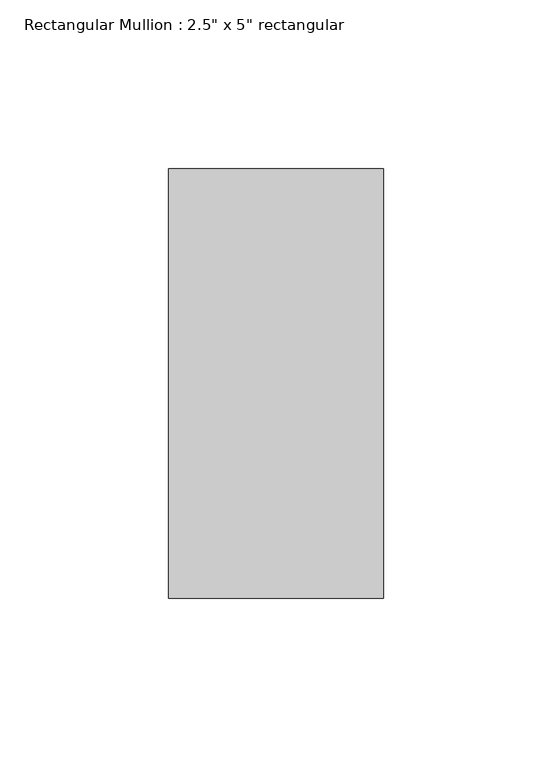
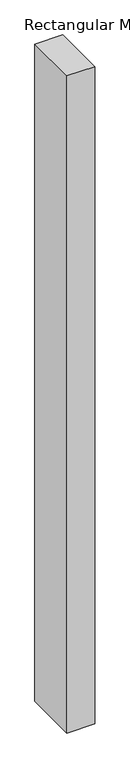
"""IFC4 building model written with IfcOpenShell, lengths in millimetres: member geometry."""

from ifc_helpers import new_model, si_unit, frame, origin, place, context, project, spatial, polyline, outline, extrude, source, transform, mapped, element, save


def member_6998075c(model_context):
    return source(origin(), model_context, "Body", "SweptSolid", [
        extrude(outline(polyline([(0.0, 63.5), (0.0, -63.5), (-63.5, -63.5), (-63.5, 63.5), (0.0, 63.5)])), frame((0.0, 0.0, -1588.1134655), z_axis=(0.0, 0.0, 1.0), x_axis=(1.0, 0.0, 0.0)), (0.0, 0.0, 1.0), 1588.1134655),
    ])


if __name__ == "__main__":
    model = new_model("IFC4")
    model_context = context("Model", 3, world=origin())
    ifc_project = project(units=[si_unit("LENGTHUNIT", "METRE", prefix="MILLI")], contexts=[model_context])
    site = spatial("IfcSite", under=ifc_project)
    building = spatial("IfcBuilding", under=site)
    placement = place(None, origin())
    member_shape = member_6998075c(model_context)
    element("IfcMember", 1, ObjectType="Rectangular Mullion : 2.5\" x 5\" rectangular", at=placement, inside=building, context=model_context, shape_type="MappedRepresentation", body=[
        mapped(member_shape, transform((0.0, 0.0, 0.0), x_axis=(1.0, 0.0, 0.0), y_axis=(0.0, 1.0, 0.0), z_axis=(0.0, 0.0, 1.0))),
    ])
    save(model, "model.ifc")

# Revit data of these elements
# Type "Rectangular Mullion : 2.5\" x 5\" rectangular"
#   built-in parameter 1007304 = 0.416667 (stored number, unit not read)
#   built-in parameter 1007301 = 0.104167 (stored number, unit not read)
#   built-in parameter 1007300 = 0.104167 (stored number, unit not read)
# Element 1 (IfcMember, "Rectangular Mullion : 2.5\" x 5\" rectangular")
#   Materials on its faces: "Aluminum"
# Materials
#   "Aluminum": class "Metal", colour RGB 247 247 247, transparency 0, Description = "Aluminum 6061", Cost = 0
